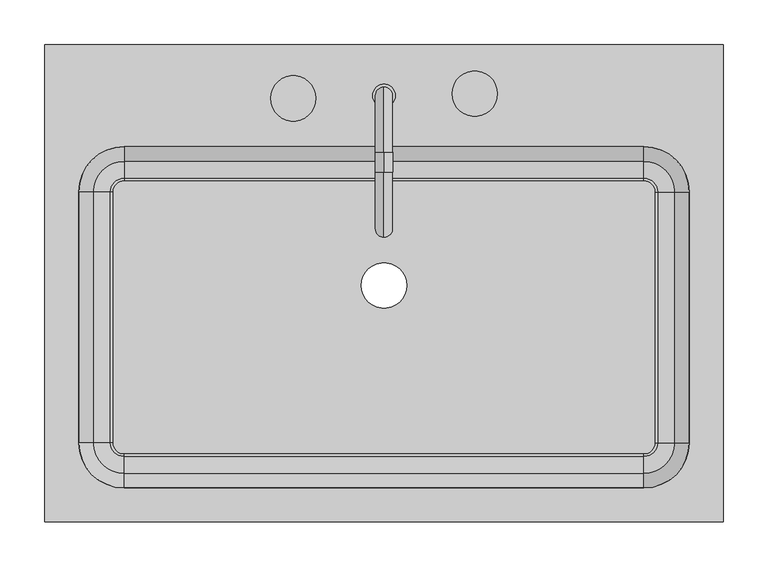
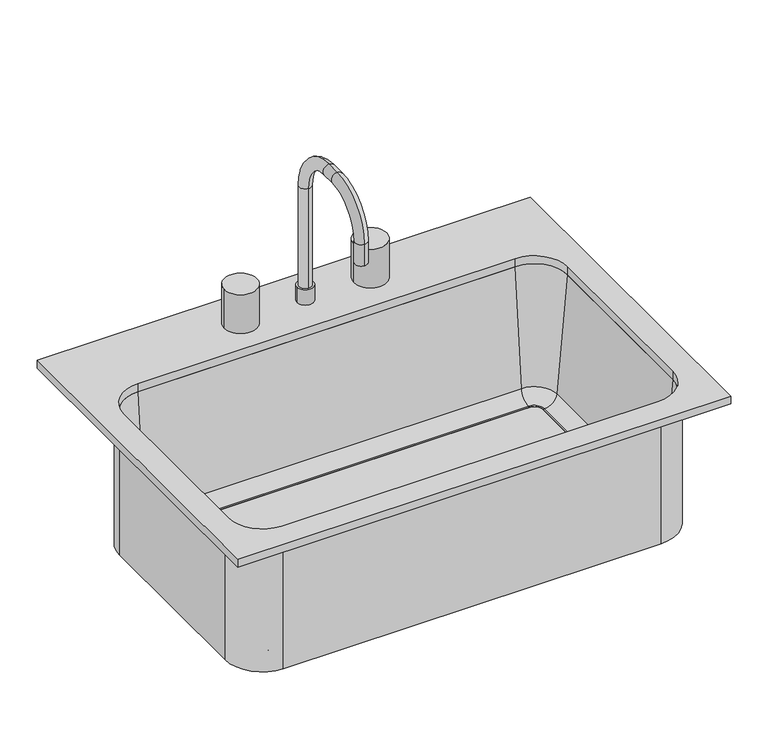
"""IFC4 building model written with IfcOpenShell, lengths in millimetres: flow terminal geometry."""

from ifc_helpers import new_model, si_unit, point, frame, frame_2d, origin, place, context, project, spatial, polyline, circle_curve, ellipse_curve, trimmed, segment, composite_curve, outline, extrude, source, transform, mapped, element, save
from ifc_brep_helpers import plane_surface, cylinder_surface, revolved_surface, advanced_brep


def flow_terminal_8307eafe(model_context):
    return source(origin(), model_context, "Body", "SolidModel", [
        extrude(outline(polyline([(395.6892406, 269.8454011), (395.6892406, -265.1545989), (-364.3107594, -265.1545989), (-364.3107594, 269.8454011), (395.6892406, 269.8454011)]), holes=[composite_curve([segment(polyline([(306.7892406, 155.5454011), (-275.4107594, 155.5454011)]), True, "CONTINUOUS"), segment(trimmed(circle_curve(frame_2d((-275.4107594, 104.7454011)), 50.8), [point((-275.4107594, 155.5454011))], [point((-326.2107594, 104.7454011))], True, "CARTESIAN"), True, "CONTINUOUS"), segment(polyline([(-326.2107594, 104.7454011), (-326.2107594, -176.2545989)]), True, "CONTINUOUS"), segment(trimmed(circle_curve(frame_2d((-275.4107594, -176.2545989)), 50.8), [point((-326.2107594, -176.2545989))], [point((-275.4107594, -227.0545989))], True, "CARTESIAN"), True, "CONTINUOUS"), segment(polyline([(-275.4107594, -227.0545989), (306.7892406, -227.0545989)]), True, "CONTINUOUS"), segment(trimmed(circle_curve(frame_2d((306.7892406, -176.2545989)), 50.8), [point((306.7892406, -227.0545989))], [point((357.5892406, -176.2545989))], True, "CARTESIAN"), True, "CONTINUOUS"), segment(polyline([(357.5892406, -176.2545989), (357.5892406, 104.7454011)]), True, "CONTINUOUS"), segment(trimmed(circle_curve(frame_2d((306.7892406, 104.7454011)), 50.8), [point((357.5892406, 104.7454011))], [point((306.7892406, 155.5454011))], True, "CARTESIAN"), True, "CONTINUOUS")], self_intersect=False)]), frame((0.0, 0.0, 900.0), z_axis=(0.0, 0.0, 1.0), x_axis=(1.0, 0.0, 0.0)), (0.0, 0.0, 1.0), 12.7),
        advanced_brep(
        [(363.9392406, 104.7454011, 684.1), (306.7892406, 161.8954011, 684.1), (306.7892406, 161.8954011, 900.0), (363.9392406, 104.7454011, 900.0), (319.4892406, 104.7454011, 684.1), (306.7892406, 117.4454011, 684.1), (319.4892406, 104.7454011, 693.625), (306.7892406, 117.4454011, 693.625), (322.0776588, 104.7454011, 693.625), (306.7892406, 120.0338193, 693.625), (341.0551678, 104.7454011, 711.0146831), (306.7892406, 139.0113283, 711.0146831), (357.5892406, 104.7454011, 900.0), (306.7892406, 155.5454011, 900.0), (363.9392406, -176.2545989, 900.0), (363.9392406, -176.2545989, 684.1), (319.4892406, -176.2545989, 684.1), (319.4892406, -176.2545989, 693.625), (322.0776588, -176.2545989, 693.625), (341.0551678, -176.2545989, 711.0146831), (357.5892406, -176.2545989, 900.0), (306.7892406, -233.4045989, 684.1), (306.7892406, -233.4045989, 900.0), (306.7892406, -188.9545989, 684.1), (306.7892406, -188.9545989, 693.625), (306.7892406, -191.5430171, 693.625), (306.7892406, -210.5205261, 711.0146831), (306.7892406, -227.0545989, 900.0), (-275.4107594, -233.4045989, 900.0), (-275.4107594, -233.4045989, 684.1), (-275.4107594, -188.9545989, 684.1), (-275.4107594, -188.9545989, 693.625), (-275.4107594, -191.5430171, 693.625), (-275.4107594, -210.5205261, 711.0146831), (-275.4107594, -227.0545989, 900.0), (-332.5607594, -176.2545989, 684.1), (-332.5607594, -176.2545989, 900.0), (-288.1107594, -176.2545989, 684.1), (-288.1107594, -176.2545989, 693.625), (-290.6991776, -176.2545989, 693.625), (-309.6766866, -176.2545989, 711.0146831), (-326.2107594, -176.2545989, 900.0), (-332.5607594, 104.7454011, 900.0), (-332.5607594, 104.7454011, 684.1), (-288.1107594, 104.7454011, 684.1), (-288.1107594, 104.7454011, 693.625), (-290.6991776, 104.7454011, 693.625), (-309.6766866, 104.7454011, 711.0146831), (-326.2107594, 104.7454011, 900.0), (-275.4107594, 161.8954011, 684.1), (-275.4107594, 161.8954011, 900.0), (-275.4107594, 117.4454011, 684.1), (-275.4107594, 117.4454011, 693.625), (-275.4107594, 120.0338193, 693.625), (-275.4107594, 139.0113283, 711.0146831), (-275.4107594, 155.5454011, 900.0)],
        [
            (0, 1, circle_curve(frame((306.7892406, 104.7454011, 684.1), z_axis=(0.0, 0.0, 1.0), x_axis=(0.0, 1.0, 0.0)), 57.15)),
            (1, 2),
            (2, 3, circle_curve(frame((306.7892406, 104.7454011, 900.0), z_axis=(0.0, 0.0, -1.0), x_axis=(0.0, 1.0, 0.0)), 57.15)),
            (3, 0),
            (4, 5, circle_curve(frame((306.7892406, 104.7454011, 684.1), z_axis=(0.0, 0.0, 1.0), x_axis=(0.0, 1.0, 0.0)), 12.7)),
            (5, 1),
            (0, 4),
            (6, 7, circle_curve(frame((306.7892406, 104.7454011, 693.625), z_axis=(0.0, 0.0, 1.0), x_axis=(0.0, 1.0, 0.0)), 12.7)),
            (7, 5),
            (4, 6),
            (8, 9, circle_curve(frame((306.7892406, 104.7454011, 693.625), z_axis=(0.0, 0.0, 1.0), x_axis=(0.0, 1.0, 0.0)), 15.2884182)),
            (9, 7),
            (6, 8),
            (10, 11, circle_curve(frame((306.7892406, 104.7454011, 711.0146831), z_axis=(0.0, 0.0, 1.0), x_axis=(0.0, 1.0, 0.0)), 34.2659272)),
            (11, 9, circle_curve(frame((306.7892406, 120.0338193, 712.675), z_axis=(-1.0, 0.0, 0.0), x_axis=(0.0, 1.0, 0.0)), 19.05)),
            (8, 10, circle_curve(frame((322.0776588, 104.7454011, 712.675), z_axis=(0.0, -1.0, 0.0), x_axis=(1.0, 0.0, 0.0)), 19.05)),
            (12, 13, circle_curve(frame((306.7892406, 104.7454011, 900.0), z_axis=(0.0, 0.0, 1.0), x_axis=(0.0, 1.0, 0.0)), 50.8)),
            (13, 11),
            (10, 12),
            (2, 13),
            (12, 3),
            (3, 14),
            (14, 15),
            (15, 0),
            (15, 16),
            (16, 4),
            (16, 17),
            (17, 6),
            (17, 18),
            (18, 8),
            (18, 19, circle_curve(frame((322.0776588, -176.2545989, 712.675), z_axis=(0.0, -1.0, 0.0), x_axis=(1.0, 0.0, 0.0)), 19.05)),
            (19, 10),
            (19, 20),
            (20, 12),
            (20, 14),
            (21, 15, circle_curve(frame((306.7892406, -176.2545989, 684.1), z_axis=(0.0, 0.0, 1.0), x_axis=(1.0, 0.0, 0.0)), 57.15)),
            (14, 22, circle_curve(frame((306.7892406, -176.2545989, 900.0), z_axis=(0.0, 0.0, -1.0), x_axis=(1.0, 0.0, 0.0)), 57.15)),
            (22, 21),
            (23, 16, circle_curve(frame((306.7892406, -176.2545989, 684.1), z_axis=(0.0, 0.0, 1.0), x_axis=(1.0, 0.0, 0.0)), 12.7)),
            (21, 23),
            (24, 17, circle_curve(frame((306.7892406, -176.2545989, 693.625), z_axis=(0.0, 0.0, 1.0), x_axis=(1.0, 0.0, 0.0)), 12.7)),
            (23, 24),
            (25, 18, circle_curve(frame((306.7892406, -176.2545989, 693.625), z_axis=(0.0, 0.0, 1.0), x_axis=(1.0, 0.0, 0.0)), 15.2884182)),
            (24, 25),
            (26, 19, circle_curve(frame((306.7892406, -176.2545989, 711.0146831), z_axis=(0.0, 0.0, 1.0), x_axis=(1.0, 0.0, 0.0)), 34.2659272)),
            (25, 26, circle_curve(frame((306.7892406, -191.5430171, 712.675), z_axis=(-1.0, 0.0, 0.0), x_axis=(0.0, -1.0, 0.0)), 19.05)),
            (27, 20, circle_curve(frame((306.7892406, -176.2545989, 900.0), z_axis=(0.0, 0.0, 1.0), x_axis=(1.0, 0.0, 0.0)), 50.8)),
            (26, 27),
            (27, 22),
            (22, 28),
            (28, 29),
            (29, 21),
            (29, 30),
            (30, 23),
            (30, 31),
            (31, 24),
            (31, 32),
            (32, 25),
            (32, 33, circle_curve(frame((-275.4107594, -191.5430171, 712.675), z_axis=(-1.0, 0.0, 0.0), x_axis=(0.0, -1.0, 0.0)), 19.05)),
            (33, 26),
            (33, 34),
            (34, 27),
            (34, 28),
            (35, 29, circle_curve(frame((-275.4107594, -176.2545989, 684.1), z_axis=(0.0, 0.0, 1.0), x_axis=(0.0, -1.0, 0.0)), 57.15)),
            (28, 36, circle_curve(frame((-275.4107594, -176.2545989, 900.0), z_axis=(0.0, 0.0, -1.0), x_axis=(0.0, -1.0, 0.0)), 57.15)),
            (36, 35),
            (37, 30, circle_curve(frame((-275.4107594, -176.2545989, 684.1), z_axis=(0.0, 0.0, 1.0), x_axis=(0.0, -1.0, 0.0)), 12.7)),
            (35, 37),
            (38, 31, circle_curve(frame((-275.4107594, -176.2545989, 693.625), z_axis=(0.0, 0.0, 1.0), x_axis=(0.0, -1.0, 0.0)), 12.7)),
            (37, 38),
            (39, 32, circle_curve(frame((-275.4107594, -176.2545989, 693.625), z_axis=(0.0, 0.0, 1.0), x_axis=(0.0, -1.0, 0.0)), 15.2884182)),
            (38, 39),
            (40, 33, circle_curve(frame((-275.4107594, -176.2545989, 711.0146831), z_axis=(0.0, 0.0, 1.0), x_axis=(0.0, -1.0, 0.0)), 34.2659272)),
            (39, 40, circle_curve(frame((-290.6991776, -176.2545989, 712.675), z_axis=(0.0, 1.0, 0.0), x_axis=(-1.0, 0.0, 0.0)), 19.05)),
            (41, 34, circle_curve(frame((-275.4107594, -176.2545989, 900.0), z_axis=(0.0, 0.0, 1.0), x_axis=(0.0, -1.0, 0.0)), 50.8)),
            (40, 41),
            (41, 36),
            (36, 42),
            (42, 43),
            (43, 35),
            (43, 44),
            (44, 37),
            (44, 45),
            (45, 38),
            (45, 46),
            (46, 39),
            (46, 47, circle_curve(frame((-290.6991776, 104.7454011, 712.675), z_axis=(0.0, 1.0, 0.0), x_axis=(-1.0, 0.0, 0.0)), 19.05)),
            (47, 40),
            (47, 48),
            (48, 41),
            (48, 42),
            (49, 43, circle_curve(frame((-275.4107594, 104.7454011, 684.1), z_axis=(0.0, 0.0, 1.0), x_axis=(-1.0, 0.0, 0.0)), 57.15)),
            (42, 50, circle_curve(frame((-275.4107594, 104.7454011, 900.0), z_axis=(0.0, 0.0, -1.0), x_axis=(-1.0, 0.0, 0.0)), 57.15)),
            (50, 49),
            (51, 44, circle_curve(frame((-275.4107594, 104.7454011, 684.1), z_axis=(0.0, 0.0, 1.0), x_axis=(-1.0, 0.0, 0.0)), 12.7)),
            (49, 51),
            (52, 45, circle_curve(frame((-275.4107594, 104.7454011, 693.625), z_axis=(0.0, 0.0, 1.0), x_axis=(-1.0, 0.0, 0.0)), 12.7)),
            (51, 52),
            (53, 46, circle_curve(frame((-275.4107594, 104.7454011, 693.625), z_axis=(0.0, 0.0, 1.0), x_axis=(-1.0, 0.0, 0.0)), 15.2884182)),
            (52, 53),
            (54, 47, circle_curve(frame((-275.4107594, 104.7454011, 711.0146831), z_axis=(0.0, 0.0, 1.0), x_axis=(-1.0, 0.0, 0.0)), 34.2659272)),
            (53, 54, circle_curve(frame((-275.4107594, 120.0338193, 712.675), z_axis=(1.0, 0.0, 0.0), x_axis=(0.0, 1.0, 0.0)), 19.05)),
            (55, 48, circle_curve(frame((-275.4107594, 104.7454011, 900.0), z_axis=(0.0, 0.0, 1.0), x_axis=(-1.0, 0.0, 0.0)), 50.8)),
            (54, 55),
            (55, 50),
            (50, 2),
            (1, 49),
            (5, 51),
            (7, 52),
            (9, 53),
            (11, 54),
            (13, 55),
        ],
        [
            cylinder_surface(frame((306.7892406, 104.7454011, 0.0), z_axis=(0.0, 0.0, -1.0), x_axis=(0.0, 1.0, 0.0)), 57.15),
            plane_surface(frame((306.7892406, 104.7454011, 684.1), z_axis=(0.0, 0.0, -1.0), x_axis=(0.0, 1.0, 0.0))),
            revolved_surface(polyline([(306.7892406, 117.4454011, 684.1), (306.7892406, 117.4454011, 693.625)]), (306.7892406, 104.7454011, 0.0), (0.0, 0.0, -1.0)),
            plane_surface(frame((306.7892406, 104.7454011, 693.625), z_axis=(0.0, 0.0, 1.0), x_axis=(0.0, 1.0, 0.0))),
            revolved_surface(trimmed(ellipse_curve(frame((306.7892406, 120.0338193, 712.675), z_axis=(1.0, 0.0, 0.0), x_axis=(0.0, 1.0, 0.0)), 19.05, 19.05), [point((306.7892406, 120.0338193, 693.625))], [point((306.7892406, 139.0113283, 711.0146831))], True, "CARTESIAN"), (306.7892406, 104.7454011, 0.0), (0.0, 0.0, -1.0)),
            revolved_surface(polyline([(306.7892406, 139.0113283, 711.0146831), (306.7892406, 155.5454011, 900.0)]), (306.7892406, 104.7454011, 0.0), (0.0, 0.0, -1.0)),
            plane_surface(frame((306.7892406, 104.7454011, 900.0), z_axis=(0.0, 0.0, 1.0), x_axis=(0.0, 1.0, 0.0))),
            plane_surface(frame((363.9392406, 104.7454011, 900.0), z_axis=(1.0, 0.0, 0.0), x_axis=(0.0, -1.0, 0.0))),
            plane_surface(frame((363.9392406, 104.7454011, 684.1), z_axis=(0.0, 0.0, -1.0), x_axis=(0.0, -1.0, 0.0))),
            plane_surface(frame((319.4892406, 104.7454011, 684.1), z_axis=(-1.0, 0.0, 0.0), x_axis=(0.0, -1.0, 0.0))),
            plane_surface(frame((319.4892406, 104.7454011, 693.625), z_axis=(0.0, 0.0, 1.0), x_axis=(0.0, -1.0, 0.0))),
            revolved_surface(polyline([(341.1276588, -176.25459890000002, 712.675), (341.1276588, 104.7454011, 712.675)]), (322.0776588, 104.7454011, 712.675), (0.0, -1.0, 0.0)),
            plane_surface(frame((341.0551678, 104.7454011, 711.0146831), z_axis=(-0.9961946980917443, 0.0, 0.08715574274767232), x_axis=(0.0, -1.0, 0.0))),
            plane_surface(frame((357.5892406, 104.7454011, 900.0), z_axis=(0.0, 0.0, 1.0), x_axis=(0.0, -1.0, 0.0))),
            cylinder_surface(frame((306.7892406, -176.2545989, 0.0), z_axis=(0.0, 0.0, -1.0), x_axis=(1.0, 0.0, 0.0)), 57.15),
            plane_surface(frame((306.7892406, -176.2545989, 684.1), z_axis=(0.0, 0.0, -1.0), x_axis=(1.0, 0.0, 0.0))),
            revolved_surface(polyline([(319.4892406, -176.2545989, 684.1), (319.4892406, -176.2545989, 693.625)]), (306.7892406, -176.2545989, 0.0), (0.0, 0.0, -1.0)),
            plane_surface(frame((306.7892406, -176.2545989, 693.625), z_axis=(0.0, 0.0, 1.0), x_axis=(1.0, 0.0, 0.0))),
            revolved_surface(trimmed(ellipse_curve(frame((322.0776588, -176.2545989, 712.675), z_axis=(0.0, -1.0, 0.0), x_axis=(1.0, 0.0, 0.0)), 19.05, 19.05), [point((322.0776588, -176.2545989, 693.625))], [point((341.0551678, -176.2545989, 711.0146831))], True, "CARTESIAN"), (306.7892406, -176.2545989, 0.0), (0.0, 0.0, -1.0)),
            revolved_surface(polyline([(341.0551678, -176.2545989, 711.0146831), (357.5892406, -176.2545989, 900.0)]), (306.7892406, -176.2545989, 0.0), (0.0, 0.0, -1.0)),
            plane_surface(frame((306.7892406, -176.2545989, 900.0), z_axis=(0.0, 0.0, 1.0), x_axis=(1.0, 0.0, 0.0))),
            plane_surface(frame((306.7892406, -233.4045989, 900.0), z_axis=(0.0, -1.0, 0.0), x_axis=(-1.0, 0.0, 0.0))),
            plane_surface(frame((306.7892406, -233.4045989, 684.1), z_axis=(0.0, 0.0, -1.0), x_axis=(-1.0, 0.0, 0.0))),
            plane_surface(frame((306.7892406, -188.9545989, 684.1), z_axis=(0.0, 1.0, 0.0), x_axis=(-1.0, 0.0, 0.0))),
            plane_surface(frame((306.7892406, -188.9545989, 693.625), z_axis=(0.0, 0.0, 1.0), x_axis=(-1.0, 0.0, 0.0))),
            revolved_surface(polyline([(-275.4107594, -210.5930171, 712.675), (306.7892406, -210.5930171, 712.675)]), (306.7892406, -191.5430171, 712.675), (-1.0, 0.0, 0.0)),
            plane_surface(frame((306.7892406, -210.5205261, 711.0146831), z_axis=(0.0, 0.9961946980917443, 0.08715574274767232), x_axis=(-1.0, 0.0, 0.0))),
            plane_surface(frame((306.7892406, -227.0545989, 900.0), z_axis=(0.0, 0.0, 1.0), x_axis=(-1.0, 0.0, 0.0))),
            cylinder_surface(frame((-275.4107594, -176.2545989, 0.0), z_axis=(0.0, 0.0, -1.0), x_axis=(0.0, -1.0, 0.0)), 57.15),
            plane_surface(frame((-275.4107594, -176.2545989, 684.1), z_axis=(0.0, 0.0, -1.0), x_axis=(0.0, -1.0, 0.0))),
            revolved_surface(polyline([(-275.4107594, -188.95459889999998, 684.1), (-275.4107594, -188.95459889999998, 693.625)]), (-275.4107594, -176.2545989, 0.0), (0.0, 0.0, -1.0)),
            plane_surface(frame((-275.4107594, -176.2545989, 693.625), z_axis=(0.0, 0.0, 1.0), x_axis=(0.0, -1.0, 0.0))),
            revolved_surface(trimmed(ellipse_curve(frame((-275.4107594, -191.5430171, 712.675), z_axis=(-1.0, 0.0, 0.0), x_axis=(0.0, -1.0, 0.0)), 19.05, 19.05), [point((-275.4107594, -191.5430171, 693.625))], [point((-275.4107594, -210.5205261, 711.0146831))], True, "CARTESIAN"), (-275.4107594, -176.2545989, 0.0), (0.0, 0.0, -1.0)),
            revolved_surface(polyline([(-275.4107594, -210.5205261, 711.0146831), (-275.4107594, -227.0545989, 900.0)]), (-275.4107594, -176.2545989, 0.0), (0.0, 0.0, -1.0)),
            plane_surface(frame((-275.4107594, -176.2545989, 900.0), z_axis=(0.0, 0.0, 1.0), x_axis=(0.0, -1.0, 0.0))),
            plane_surface(frame((-332.5607594, -176.2545989, 900.0), z_axis=(-1.0, 0.0, 0.0), x_axis=(0.0, 1.0, 0.0))),
            plane_surface(frame((-332.5607594, -176.2545989, 684.1), z_axis=(0.0, 0.0, -1.0), x_axis=(0.0, 1.0, 0.0))),
            plane_surface(frame((-288.1107594, -176.2545989, 684.1), z_axis=(1.0, 0.0, 0.0), x_axis=(0.0, 1.0, 0.0))),
            plane_surface(frame((-288.1107594, -176.2545989, 693.625), z_axis=(0.0, 0.0, 1.0), x_axis=(0.0, 1.0, 0.0))),
            revolved_surface(polyline([(-309.7491776, 104.74540110000001, 712.675), (-309.7491776, -176.2545989, 712.675)]), (-290.6991776, -176.2545989, 712.675), (0.0, 1.0, 0.0)),
            plane_surface(frame((-309.6766866, -176.2545989, 711.0146831), z_axis=(0.9961946980917443, 0.0, 0.08715574274767232), x_axis=(0.0, 1.0, 0.0))),
            plane_surface(frame((-326.2107594, -176.2545989, 900.0), z_axis=(0.0, 0.0, 1.0), x_axis=(0.0, 1.0, 0.0))),
            cylinder_surface(frame((-275.4107594, 104.7454011, 0.0), z_axis=(0.0, 0.0, -1.0), x_axis=(-1.0, 0.0, 0.0)), 57.15),
            plane_surface(frame((-275.4107594, 104.7454011, 684.1), z_axis=(0.0, 0.0, -1.0), x_axis=(-1.0, 0.0, 0.0))),
            revolved_surface(polyline([(-288.1107594, 104.7454011, 684.1), (-288.1107594, 104.7454011, 693.625)]), (-275.4107594, 104.7454011, 0.0), (0.0, 0.0, -1.0)),
            plane_surface(frame((-275.4107594, 104.7454011, 693.625), z_axis=(0.0, 0.0, 1.0), x_axis=(-1.0, 0.0, 0.0))),
            revolved_surface(trimmed(ellipse_curve(frame((-290.6991776, 104.7454011, 712.675), z_axis=(0.0, 1.0, 0.0), x_axis=(-1.0, 0.0, 0.0)), 19.05, 19.05), [point((-290.6991776, 104.7454011, 693.625))], [point((-309.6766866, 104.7454011, 711.0146831))], True, "CARTESIAN"), (-275.4107594, 104.7454011, 0.0), (0.0, 0.0, -1.0)),
            revolved_surface(polyline([(-309.6766866, 104.7454011, 711.0146831), (-326.2107594, 104.7454011, 900.0)]), (-275.4107594, 104.7454011, 0.0), (0.0, 0.0, -1.0)),
            plane_surface(frame((-275.4107594, 104.7454011, 900.0), z_axis=(0.0, 0.0, 1.0), x_axis=(-1.0, 0.0, 0.0))),
            plane_surface(frame((-275.4107594, 161.8954011, 900.0), z_axis=(0.0, 1.0, 0.0), x_axis=(1.0, 0.0, 0.0))),
            plane_surface(frame((-275.4107594, 161.8954011, 684.1), z_axis=(0.0, 0.0, -1.0), x_axis=(1.0, 0.0, 0.0))),
            plane_surface(frame((-275.4107594, 117.4454011, 684.1), z_axis=(0.0, -1.0, 0.0), x_axis=(1.0, 0.0, 0.0))),
            plane_surface(frame((-275.4107594, 117.4454011, 693.625), z_axis=(0.0, 0.0, 1.0), x_axis=(1.0, 0.0, 0.0))),
            revolved_surface(polyline([(306.7892406, 139.08381930000002, 712.675), (-275.4107594, 139.08381930000002, 712.675)]), (-275.4107594, 120.0338193, 712.675), (1.0, 0.0, 0.0)),
            plane_surface(frame((-275.4107594, 139.0113283, 711.0146831), z_axis=(0.0, -0.9961946980917443, 0.08715574274767232), x_axis=(1.0, 0.0, 0.0))),
            plane_surface(frame((-275.4107594, 155.5454011, 900.0), z_axis=(0.0, 0.0, 1.0), x_axis=(1.0, 0.0, 0.0))),
        ],
        [
            (0, [[1, 2, 3, 4]]),
            (1, [[5, 6, -1, 7]]),
            (2, [[8, 9, -5, 10]]),
            (3, [[11, 12, -8, 13]]),
            (4, [[14, 15, -11, 16]]),
            (5, [[17, 18, -14, 19]]),
            (6, [[-3, 20, -17, 21]]),
            (7, [[-4, 22, 23, 24]]),
            (8, [[-7, -24, 25, 26]]),
            (9, [[-10, -26, 27, 28]]),
            (10, [[-13, -28, 29, 30]]),
            (11, [[-16, -30, 31, 32]]),
            (12, [[-19, -32, 33, 34]]),
            (13, [[-21, -34, 35, -22]]),
            (14, [[36, -23, 37, 38]]),
            (15, [[39, -25, -36, 40]]),
            (16, [[41, -27, -39, 42]]),
            (17, [[43, -29, -41, 44]]),
            (18, [[45, -31, -43, 46]]),
            (19, [[47, -33, -45, 48]]),
            (20, [[-37, -35, -47, 49]]),
            (21, [[-38, 50, 51, 52]]),
            (22, [[-40, -52, 53, 54]]),
            (23, [[-42, -54, 55, 56]]),
            (24, [[-44, -56, 57, 58]]),
            (25, [[-46, -58, 59, 60]]),
            (26, [[-48, -60, 61, 62]]),
            (27, [[-49, -62, 63, -50]]),
            (28, [[64, -51, 65, 66]]),
            (29, [[67, -53, -64, 68]]),
            (30, [[69, -55, -67, 70]]),
            (31, [[71, -57, -69, 72]]),
            (32, [[73, -59, -71, 74]]),
            (33, [[75, -61, -73, 76]]),
            (34, [[-65, -63, -75, 77]]),
            (35, [[-66, 78, 79, 80]]),
            (36, [[-68, -80, 81, 82]]),
            (37, [[-70, -82, 83, 84]]),
            (38, [[-72, -84, 85, 86]]),
            (39, [[-74, -86, 87, 88]]),
            (40, [[-76, -88, 89, 90]]),
            (41, [[-77, -90, 91, -78]]),
            (42, [[92, -79, 93, 94]]),
            (43, [[95, -81, -92, 96]]),
            (44, [[97, -83, -95, 98]]),
            (45, [[99, -85, -97, 100]]),
            (46, [[101, -87, -99, 102]]),
            (47, [[103, -89, -101, 104]]),
            (48, [[-93, -91, -103, 105]]),
            (49, [[-94, 106, -2, 107]]),
            (50, [[-96, -107, -6, 108]]),
            (51, [[-98, -108, -9, 109]]),
            (52, [[-100, -109, -12, 110]]),
            (53, [[-102, -110, -15, 111]]),
            (54, [[-104, -111, -18, 112]]),
            (55, [[-105, -112, -20, -106]]),
        ],
    ),
        extrude(outline(composite_curve([segment(trimmed(circle_curve(frame_2d((306.7892406, 104.7454011)), 12.7), [point((306.7892406, 117.4454011))], [point((319.4892406, 104.7454011))], False, "CARTESIAN"), True, "CONTINUOUS"), segment(polyline([(319.4892406, 104.7454011), (319.4892406, -176.2545989)]), True, "CONTINUOUS"), segment(trimmed(circle_curve(frame_2d((306.7892406, -176.2545989)), 12.7), [point((319.4892406, -176.2545989))], [point((306.7892406, -188.9545989))], False, "CARTESIAN"), True, "CONTINUOUS"), segment(polyline([(306.7892406, -188.9545989), (-275.4107594, -188.9545989)]), True, "CONTINUOUS"), segment(trimmed(circle_curve(frame_2d((-275.4107594, -176.2545989)), 12.7), [point((-275.4107594, -188.9545989))], [point((-288.1107594, -176.2545989))], False, "CARTESIAN"), True, "CONTINUOUS"), segment(polyline([(-288.1107594, -176.2545989), (-288.1107594, 104.7454011)]), True, "CONTINUOUS"), segment(trimmed(circle_curve(frame_2d((-275.4107594, 104.7454011)), 12.7), [point((-288.1107594, 104.7454011))], [point((-275.4107594, 117.4454011))], False, "CARTESIAN"), True, "CONTINUOUS"), segment(polyline([(-275.4107594, 117.4454011), (306.7892406, 117.4454011)]), True, "CONTINUOUS")], self_intersect=False), holes=[composite_curve([segment(trimmed(circle_curve(frame_2d((15.6892406, 0.0)), 25.4), [point((-9.7107594, 0.0))], [point((41.0892406, 0.0))], True, "CARTESIAN"), True, "CONTINUOUS"), segment(trimmed(circle_curve(frame_2d((15.6892406, 0.0)), 25.4), [point((41.0892406, 0.0))], [point((-9.7107594, 0.0))], True, "CARTESIAN"), True, "CONTINUOUS")], self_intersect=False)]), frame((0.0, 0.0, 684.1), z_axis=(0.0, 0.0, 1.0), x_axis=(1.0, 0.0, 0.0)), (0.0, 0.0, 1.0), 9.525),
        extrude(outline(composite_curve([segment(trimmed(circle_curve(frame_2d((-85.9107594, 209.6166076)), 25.4), [point((-111.3107594, 209.6166076))], [point((-60.5107594, 209.6166076))], False, "CARTESIAN"), True, "CONTINUOUS"), segment(trimmed(circle_curve(frame_2d((-85.9107594, 209.6166076)), 25.4), [point((-60.5107594, 209.6166076))], [point((-111.3107594, 209.6166076))], False, "CARTESIAN"), True, "CONTINUOUS")], self_intersect=False)), frame((0.0, 0.0, 912.7), z_axis=(0.0, 0.0, 1.0), x_axis=(1.0, 0.0, 0.0)), (0.0, 0.0, 1.0), 63.5),
        extrude(outline(composite_curve([segment(trimmed(circle_curve(frame_2d((117.2892406, 214.8133323)), 25.4), [point((91.8892406, 214.8133323))], [point((142.6892406, 214.8133323))], False, "CARTESIAN"), True, "CONTINUOUS"), segment(trimmed(circle_curve(frame_2d((117.2892406, 214.8133323)), 25.4), [point((142.6892406, 214.8133323))], [point((91.8892406, 214.8133323))], False, "CARTESIAN"), True, "CONTINUOUS")], self_intersect=False)), frame((0.0, 0.0, 912.7), z_axis=(0.0, 0.0, 1.0), x_axis=(1.0, 0.0, 0.0)), (0.0, 0.0, 1.0), 63.5),
        advanced_brep(
        [(15.6892406, 222.2204011, 912.7), (15.6892406, 203.1704011, 912.7), (15.6892406, 222.2204011, 1100.025), (15.6892406, 203.1704011, 1100.025), (15.6892406, 149.1954011, 1154.0), (15.6892406, 149.1954011, 1173.05), (15.6892406, 126.9704011, 1173.05), (15.6892406, 126.9704011, 1154.0), (15.6892406, 72.9954011, 1100.025), (15.6892406, 53.9454011, 1100.025), (15.6892406, 53.9454011, 1065.1), (15.6892406, 72.9954011, 1065.1)],
        [
            (0, 1, circle_curve(frame((15.6892406, 212.6954011, 912.7), z_axis=(0.0, 0.0, -1.0), x_axis=(0.0, -1.0, 0.0)), 9.525)),
            (1, 0, circle_curve(frame((15.6892406, 212.6954011, 912.7), z_axis=(0.0, 0.0, -1.0), x_axis=(0.0, -1.0, 0.0)), 9.525)),
            (0, 2),
            (2, 3, circle_curve(frame((15.6892406, 212.6954011, 1100.025), z_axis=(0.0, 0.0, -1.0), x_axis=(0.0, -1.0, 0.0)), 9.525)),
            (3, 1),
            (3, 2, circle_curve(frame((15.6892406, 212.6954011, 1100.025), z_axis=(0.0, 0.0, -1.0), x_axis=(0.0, -1.0, 0.0)), 9.525)),
            (4, 3, circle_curve(frame((15.6892406, 149.1954011, 1100.025), z_axis=(-1.0, 0.0, 0.0), x_axis=(0.0, 1.0, 0.0)), 53.975)),
            (2, 5, circle_curve(frame((15.6892406, 149.1954011, 1100.025), z_axis=(1.0, 0.0, 0.0), x_axis=(0.0, 1.0, 0.0)), 73.025)),
            (5, 4, circle_curve(frame((15.6892406, 149.1954011, 1163.525), z_axis=(0.0, 1.0, 0.0), x_axis=(0.0, 0.0, -1.0)), 9.525)),
            (4, 5, circle_curve(frame((15.6892406, 149.1954011, 1163.525), z_axis=(0.0, 1.0, 0.0), x_axis=(0.0, 0.0, -1.0)), 9.525)),
            (5, 6),
            (6, 7, circle_curve(frame((15.6892406, 126.9704011, 1163.525), z_axis=(0.0, 1.0, 0.0), x_axis=(0.0, 0.0, -1.0)), 9.525)),
            (7, 4),
            (7, 6, circle_curve(frame((15.6892406, 126.9704011, 1163.525), z_axis=(0.0, 1.0, 0.0), x_axis=(0.0, 0.0, -1.0)), 9.525)),
            (8, 7, circle_curve(frame((15.6892406, 126.9704011, 1100.025), z_axis=(-1.0, 0.0, 0.0), x_axis=(0.0, 0.0, 1.0)), 53.975)),
            (6, 9, circle_curve(frame((15.6892406, 126.9704011, 1100.025), z_axis=(1.0, 0.0, 0.0), x_axis=(0.0, 0.0, 1.0)), 73.025)),
            (9, 8, circle_curve(frame((15.6892406, 63.4704011, 1100.025), z_axis=(0.0, 0.0, 1.0), x_axis=(0.0, 1.0, 0.0)), 9.525)),
            (8, 9, circle_curve(frame((15.6892406, 63.4704011, 1100.025), z_axis=(0.0, 0.0, 1.0), x_axis=(0.0, 1.0, 0.0)), 9.525)),
            (10, 11, circle_curve(frame((15.6892406, 63.4704011, 1065.1), z_axis=(0.0, 0.0, -1.0), x_axis=(0.0, 1.0, 0.0)), 9.525)),
            (11, 10, circle_curve(frame((15.6892406, 63.4704011, 1065.1), z_axis=(0.0, 0.0, -1.0), x_axis=(0.0, 1.0, 0.0)), 9.525)),
            (9, 10),
            (11, 8),
        ],
        [
            plane_surface(frame((15.6892406, 203.1704011, 912.7), z_axis=(0.0, 0.0, -1.0), x_axis=(1.0, 0.0, 0.0))),
            cylinder_surface(frame((15.6892406, 212.6954011, 912.7), z_axis=(0.0, 0.0, -1.0), x_axis=(0.0, -1.0, 0.0)), 9.525),
            revolved_surface(trimmed(ellipse_curve(frame((15.6892406, 212.6954011, 1100.025), z_axis=(0.0, 0.0, -1.0), x_axis=(0.0, -1.0, 0.0)), 9.525, 9.525), [point((15.6892406, 222.2204011, 1100.025))], [point((15.6892406, 203.1704011, 1100.025))], True, "CARTESIAN"), (15.6892406, 149.1954011, 1100.025), (1.0, 0.0, 0.0)),
            revolved_surface(trimmed(ellipse_curve(frame((15.6892406, 212.6954011, 1100.025), z_axis=(0.0, 0.0, -1.0), x_axis=(0.0, -1.0, 0.0)), 9.525, 9.525), [point((15.6892406, 203.1704011, 1100.025))], [point((15.6892406, 222.2204011, 1100.025))], True, "CARTESIAN"), (15.6892406, 149.1954011, 1100.025), (1.0, 0.0, 0.0)),
            cylinder_surface(frame((15.6892406, 149.1954011, 1163.525), z_axis=(0.0, 1.0, 0.0), x_axis=(0.0, 0.0, -1.0)), 9.525),
            revolved_surface(trimmed(ellipse_curve(frame((15.6892406, 126.9704011, 1163.525), z_axis=(0.0, 1.0, 0.0), x_axis=(0.0, 0.0, -1.0)), 9.525, 9.525), [point((15.6892406, 126.9704011, 1173.05))], [point((15.6892406, 126.9704011, 1154.0))], True, "CARTESIAN"), (15.6892406, 126.9704011, 1100.025), (1.0, 0.0, 0.0)),
            revolved_surface(trimmed(ellipse_curve(frame((15.6892406, 126.9704011, 1163.525), z_axis=(0.0, 1.0, 0.0), x_axis=(0.0, 0.0, -1.0)), 9.525, 9.525), [point((15.6892406, 126.9704011, 1154.0))], [point((15.6892406, 126.9704011, 1173.05))], True, "CARTESIAN"), (15.6892406, 126.9704011, 1100.025), (1.0, 0.0, 0.0)),
            plane_surface(frame((15.6892406, 53.9454011, 1065.1), z_axis=(0.0, 0.0, -1.0), x_axis=(-1.0, 0.0, 0.0))),
            cylinder_surface(frame((15.6892406, 63.4704011, 1100.025), z_axis=(0.0, 0.0, 1.0), x_axis=(0.0, 1.0, 0.0)), 9.525),
        ],
        [
            (0, [[1, 2]]),
            (1, [[-1, 3, 4, 5]]),
            (1, [[-2, -5, 6, -3]]),
            (2, [[7, -4, 8, 9]]),
            (3, [[-8, -6, -7, 10]]),
            (4, [[-9, 11, 12, 13]]),
            (4, [[-10, -13, 14, -11]]),
            (5, [[15, -12, 16, 17]]),
            (6, [[-16, -14, -15, 18]]),
            (7, [[19, 20]]),
            (8, [[-17, 21, -20, 22]]),
            (8, [[-18, -22, -19, -21]]),
        ],
    ),
        extrude(outline(composite_curve([segment(trimmed(circle_curve(frame_2d((15.6892406, 212.6954011)), 12.7), [point((2.9892406, 212.6954011))], [point((28.3892406, 212.6954011))], False, "CARTESIAN"), True, "CONTINUOUS"), segment(trimmed(circle_curve(frame_2d((15.6892406, 212.6954011)), 12.7), [point((28.3892406, 212.6954011))], [point((2.9892406, 212.6954011))], False, "CARTESIAN"), True, "CONTINUOUS")], self_intersect=False)), frame((0.0, 0.0, 912.7), z_axis=(0.0, 0.0, 1.0), x_axis=(1.0, 0.0, 0.0)), (0.0, 0.0, 1.0), 25.4),
    ])


if __name__ == "__main__":
    model = new_model("IFC4")
    model_context = context("Model", 3, world=origin())
    ifc_project = project(units=[si_unit("LENGTHUNIT", "METRE", prefix="MILLI")], contexts=[model_context])
    site = spatial("IfcSite", under=ifc_project)
    building = spatial("IfcBuilding", under=site)
    placement = place(None, origin())
    flow_terminal_shape = flow_terminal_8307eafe(model_context)
    element("IfcFlowTerminal", 1, at=placement, inside=building, context=model_context, shape_type="MappedRepresentation", body=[
        mapped(flow_terminal_shape, transform((0.0, 0.0, 0.0), x_axis=(1.0, 0.0, 0.0), y_axis=(0.0, 1.0, 0.0), z_axis=(0.0, 0.0, 1.0))),
    ])
    save(model, "model.ifc")

# Revit data of these elements
# Type
#   Hauteur du plan de travail = 2.952756 ft
#   Profondeur = 1.755249 ft
#   Largeur = 2.493438 ft
#   Default Elevation = 0
